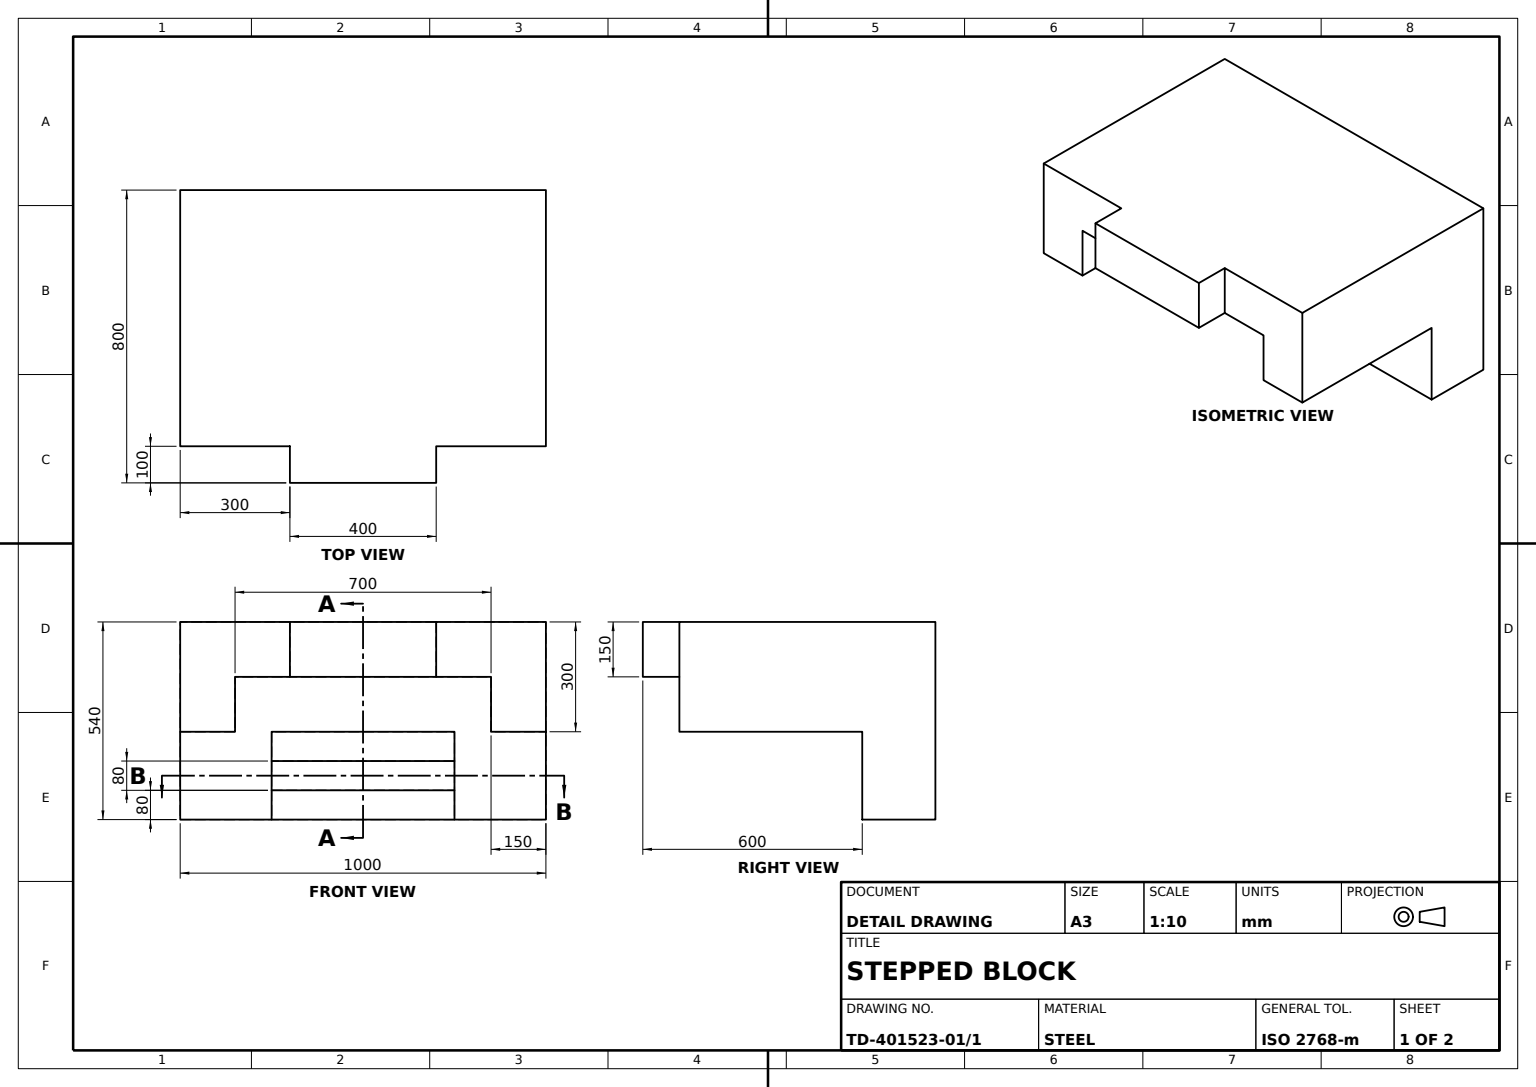
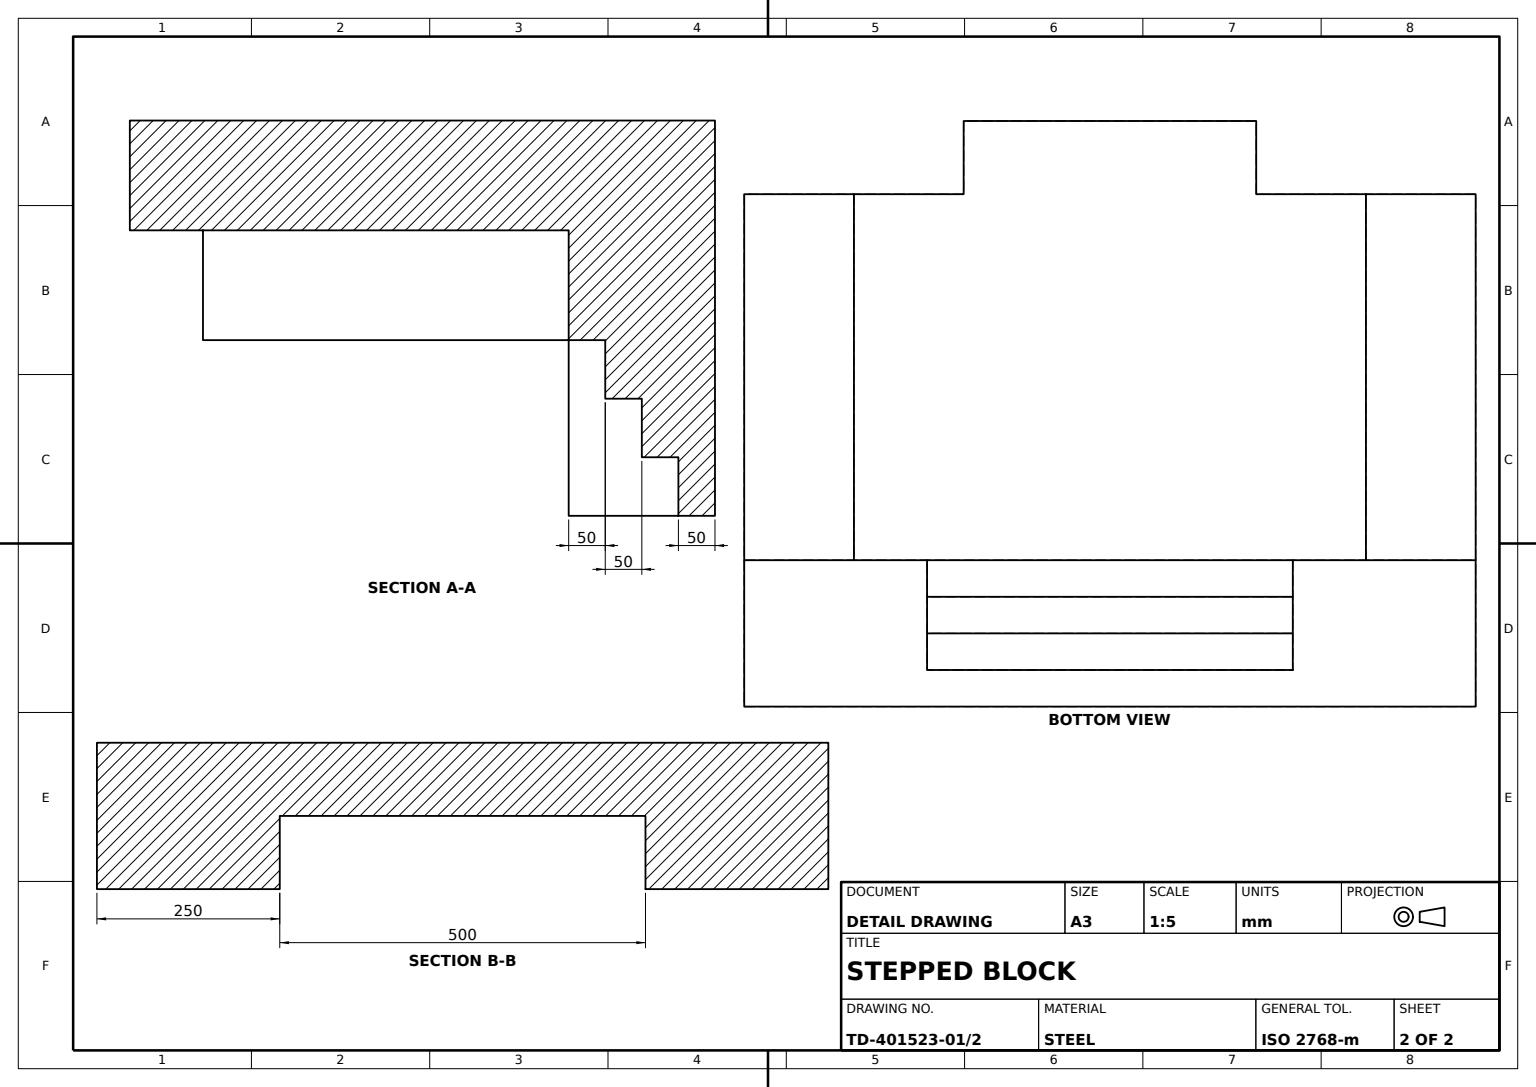
SolidWorks part; units mm, degrees
material "Plain Carbon Steel"
ref_plane "Front Plane" through (0, 0, 0) normal (0, 0, 1) x (1, 0, 0)
ref_plane "Top Plane" through (0, 0, 0) normal (0, 1, 0) x (1, 0, 0)
ref_plane "Right Plane" through (0, 0, 0) normal (1, 0, 0) x (0, 0, -1)
sketch "Base Block Profile" plane through (0, 0, 0) normal (0, 0, 1) x (1, 0, 0)
  line L0 (0, 0) -> (1000, 0)
  line L1 (1000, 0) -> (1000, 540)
  line L2 (1000, 540) -> (0, 540)
  line L3 (0, 540) -> (0, 0)
  dimension "D1" = 1000
  dimension "D2" = 540
  dimension "D3" = 1000
extrude "Base Block" add sketch "Base Block Profile" along normal blind 200
sketch "Raised Block Profile" plane through (1000, 0, 0) normal (1, 0, 0) x (0, 0, -1)
  line L0 (-200, 540) -> (-800, 540)
  line L1 (-800, 540) -> (-800, 240)
  line L2 (-800, 240) -> (-200, 240)
  line L3 (-200, 0) -> (-200, 540) construction
  line L4 (-200, 240) -> (-200, 540)
  dimension "D1" = 600
  dimension "D2" = 300
extrude "Raised Block" add sketch "Raised Block Profile" against normal blind 1000
sketch "Raised Block Step Cut Profile" plane through (0, 0, 800) normal (0, 0, 1) x (1, 0, 0)
  line L0 (0, 540) -> (0, 240)
  line L1 (0, 240) -> (1000, 240)
  line L2 (1000, 240) -> (1000, 540)
  line L3 (1000, 540) -> (0, 540)
extrude "Raised Block Step Cut" cut sketch "Raised Block Step Cut Profile" against normal blind 100
sketch "Stair Step Boss Profile" plane through (0, 540, 0) normal (0, 1, 0) x (1, 0, 0)
  line L0 (500, -700) -> (500, -800)
  line L1 (1000, -700) -> (0, -700) construction
  line L2 (500, -800) -> (700, -800)
  line L3 (700, -800) -> (700, -700)
  line L4 (700, -700) -> (300, -700)
  line L5 (300, -700) -> (300, -800)
  line L6 (300, -800) -> (500, -800)
  line M1 (0, -700) -> (1000, -700)
  dimension "D1" = 100
  dimension "D2" = 200
  dimension "D3" = 400
  dimension "D4" = 100
extrude "Stair Step Boss" add sketch "Stair Step Boss Profile" against normal blind 150 contours L5 L6 L0 M1 | L2 L3 L0 M1
sketch "Stair Cutout Profile" plane through (0, 240, 0) normal (0, -1, 0) x (1, 0, 0)
  line L0 (0, 700) -> (1000, 700) construction
  line L1 (500, 700) -> (150, 700)
  line L2 (150, 700) -> (150, 200)
  line L3 (0, 200) -> (1000, 200) construction
  line L4 (150, 200) -> (850, 200)
  line L5 (0, 200) -> (1000, 200) construction
  line L6 (850, 200) -> (850, 700)
  line L7 (850, 700) -> (500, 700)
  dimension "D1" = 350
  dimension "D2" = 700
extrude "Stair Cutout" cut sketch "Stair Cutout Profile" against normal blind 150
sketch "Stepped Slot Profile" plane through (0, 0, 200) normal (0, 0, 1) x (1, 0, 0)
  line L0 (500, 0) -> (500, 80)
  line L1 (0, 0) -> (1000, 0) construction
  line L2 (500, 80) -> (750, 80)
  line L3 (750, 80) -> (750, 0)
  line L4 (750, 0) -> (250, 0)
  line L5 (250, 0) -> (250, 80)
  line L6 (250, 80) -> (500, 80)
  line M3 (0, 0) -> (1000, 0)
  dimension "D1" = 80
  dimension "D2" = 250
  dimension "D3" = 80
  dimension "D4" = 500
  dimension "D5" = 80
extrude "Stepped Slot Cut" cut sketch "Stepped Slot Profile" against normal blind 150 contours L6 L5 L0 M3 | L3 L2 L0 M3
sketch "Slot Second Step Profile" plane through (0, 0, 200) normal (0, 0, 1) x (1, 0, 0)
  line L0 (250, 80) -> (250, 160)
  line L1 (250, 160) -> (750, 160)
  line L2 (750, 160) -> (750, 80)
  line L3 (750, 80) -> (250, 80)
  line L6 (700, 390) -> (700, 540) construction
  point P6 (750, 120)
  dimension "D1" = 80
  dimension "D2" = 500
  dimension "D3" = 50
extrude "Slot Second Step Cut" cut sketch "Slot Second Step Profile" against normal blind 100
sketch "Slot Third Step Profile" plane through (0, 0, 200) normal (0, 0, 1) x (1, 0, 0)
  line L0 (250, 160) -> (250, 240)
  line L1 (250, 240) -> (750, 240)
  line L2 (750, 240) -> (750, 160)
  line L3 (750, 160) -> (250, 160)
  dimension "D1" = 80
  dimension "D2" = 500
  dimension "D3" = 80
extrude "Slot Third Step Cut" cut sketch "Slot Third Step Profile" against normal blind 50
